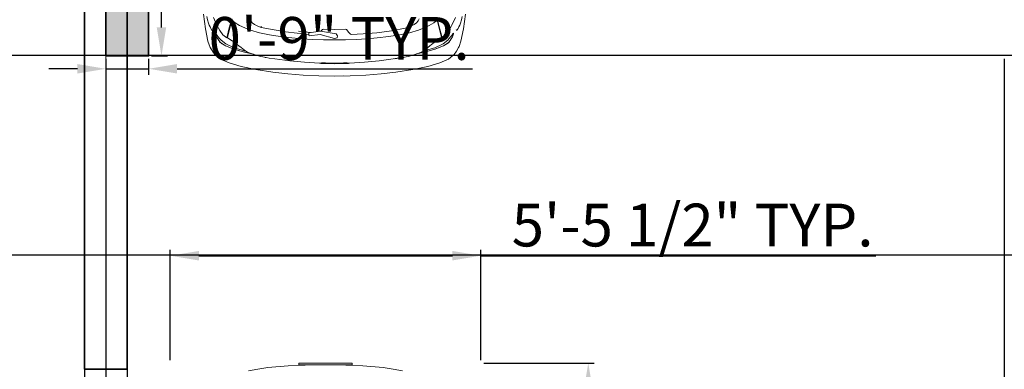
# Model space of a CAD drawing. Units: millimetres. Extents: x 595116 to 630915, y 909473 to 920225.
# Tile 113 of 134: x 629298 to 629505, y 919346 to 919419. Entities that reach past the tile are written whole.
import ezdxf

# ---------------------------------------------------------------- set-up
doc = ezdxf.new("R2010")
doc.units = ezdxf.units.MM
doc.linetypes.add('ACAD_ISO02W100', pattern=[15, 12, -3])
for name, color, linetype, lineweight in [('A-FLOR-OVHD', 253, 'ACAD_ISO02W100', 13), ('A-WALL', 1, 'Continuous', 35), ('C-PRKG-VEHI', 8, 'Continuous', 13), ('C-PROP', 7, 'Continuous', 25), ('C-PROP-REF', 240, 'ACAD_ISO02W100', 13), ('Column', 6, 'Continuous', 35), ('Dimension', 3, 'Continuous', 18)]:
    doc.layers.add(name, color=color, linetype=linetype, lineweight=lineweight)
doc.styles.get("Standard").update_dxf_attribs({"font": 'arial.ttf'})
doc.dimstyles.new('ISO-25', dxfattribs={"dimtxt": 9, "dimasz": 6, "dimexe": 1.25, "dimexo": 0.625, "dimtad": 1, "dimlunit": 4, "dimtxsty": 'Standard', "dimcen": 2.5, "dimadec": 0, "dimazin": 0, "dimtfac": 1, "dimtmove": 0, "dimatfit": 3, "dimfxl": 1, "dimarcsym": 0})

# ---------------------------------------------------------------- blocks, each defined once
blk = doc.blocks.new('A$C7ADB3080')
for p, q in [((4202.8, 1787.5), (4110.6, 1799.9)), ((4145.5, 1773.8), (4125.1, 1778.5)), ((4180, 1714.9), (4131.6, 1736.2)), ((4166.8, 1768.8), (4145.5, 1773.8)), ((4179.6, 1763.4), (4166.8, 1768.8)), ((4190.3, 1758.6), (4179.6, 1763.4)), ((4201, 1753), (4190.3, 1758.6)), ((4208.9, 1748.3), (4201, 1753)), ((4281.2, 1771.5), (4202.8, 1787.5)), ((4208.9, 1748.3), (4210.6, 1746.2)), ((4208.9, 1742.4), (4210.6, 1746.2)), ((4211.3, 1742.1), (4209, 1742.8)), ((4210, 1745), (4210.4, 1744.8)), ((4210.4, 1744.8), (4211.4, 1741.7)), ((4314.2, 1759.2), (4281.2, 1771.5)), ((4314.2, 1759.2), (4319.2, 1756.8)), ((4343.6, 1743.2), (4319.2, 1756.8)), ((4343.6, 1743.2), (4363.1, 1729.2)), ((4213.7, 1697), (4180, 1714.9)), ((4239.6, 1677.1), (4213.7, 1697)), ((4230.6, 1723.8), (4234.6, 1720.4)), ((4233.3, 1723.8), (4230.6, 1723.8)), ((4234.6, 1720.4), (4230.6, 1723.8)), ((4230.6, 1723.8), (4233.3, 1723.8)), ((4246.7, 1719.9), (4233.3, 1723.8)), ((4233.3, 1723.8), (4246.7, 1719.9)), ((4234.6, 1720.4), (4245.3, 1713.2)), ((4245.3, 1713.2), (4234.6, 1720.4)), ((4260.4, 1652.9), (4239.6, 1677.1)), ((4245.3, 1713.2), (4253.1, 1706.5)), ((4253.1, 1706.5), (4245.3, 1713.2)), ((4252.8, 1717.5), (4246.7, 1719.9)), ((4246.7, 1719.9), (4252.8, 1717.5)), ((4259.8, 1713.6), (4252.8, 1717.5)), ((4252.8, 1717.5), (4259.8, 1713.6)), ((4253.1, 1706.5), (4263.7, 1698)), ((4263.7, 1698), (4253.1, 1706.5)), ((4266.7, 1709.2), (4259.8, 1713.6)), ((4259.8, 1713.6), (4266.7, 1709.2)), ((4263.7, 1698), (4274.7, 1689.4)), ((4274.7, 1689.4), (4263.7, 1698)), ((4275.4, 1703.2), (4266.7, 1709.2)), ((4266.7, 1709.2), (4275.4, 1703.2)), ((4274.7, 1689.4), (4297.1, 1658.8)), ((4297.1, 1658.8), (4274.7, 1689.4)), ((4287.1, 1694.7), (4275.4, 1703.2)), ((4275.4, 1703.2), (4287.1, 1694.7)), ((4288.8, 1695.5), (4283, 1700)), ((4290.4, 1690), (4287.1, 1694.7)), ((4287.1, 1694.7), (4290.4, 1690)), ((4310.5, 1661.7), (4290.3, 1693.3)), ((4301.5, 1673.7), (4290.4, 1690)), ((4290.4, 1690), (4301.5, 1673.7)), ((4309.4, 1661.5), (4301.5, 1673.7)), ((4301.5, 1673.7), (4309.4, 1661.5)), ((4370.3, 1721.1), (4363.1, 1729.2)), ((4370.3, 1721.1), (4392.6, 1692.2)), ((4392.6, 1692.2), (4416.8, 1638.5)), ((4146.3, 1623.6), (4139.4, 1620.9)), ((4146.3, 1623.6), (4164.8, 1600.2)), ((4146.5, 1623.3), (4204.9, 1639.5)), ((4204.1, 1635.6), (4147.6, 1621.9)), ((4248.1, 1646.9), (4204.1, 1635.6)), ((4204.9, 1639.5), (4250.9, 1650.7)), ((4246.7, 1649.7), (4249, 1647.1)), ((4256.1, 1648.5), (4248.1, 1646.9)), ((4250.9, 1650.7), (4260.4, 1652.9)), ((4254.1, 1651.5), (4256.3, 1648.9)), ((4256.5, 1648.5), (4256.1, 1648.5)), ((4256.3, 1648.9), (4256.6, 1648.3)), ((4259.7, 1648.5), (4257.4, 1648.5)), ((4278, 1619.2), (4259.7, 1648.5)), ((4289.5, 1603), (4278, 1619.2)), ((4297.1, 1658.8), (4321.2, 1607.2)), ((4321.2, 1607.2), (4297.1, 1658.8)), ((4316, 1644.7), (4309.4, 1661.5)), ((4309.4, 1661.5), (4316, 1644.7)), ((4330.7, 1608.4), (4310.5, 1661.7)), ((4330, 1607.9), (4316, 1644.7)), ((4316, 1644.7), (4330, 1607.9)), ((4416.8, 1638.5), (4439, 1562.7)), ((4164.8, 1600.2), (4181.7, 1572.2)), ((4181.7, 1572.2), (4196.9, 1540)), ((4295.4, 1594.5), (4289.5, 1603)), ((4301.5, 1587.2), (4295.4, 1594.5)), ((4309, 1576.5), (4301.5, 1587.2)), ((4319.8, 1563.6), (4309, 1576.5)), ((4337.2, 1542.2), (4319.8, 1563.6)), ((4321.2, 1607.2), (4337.1, 1555.5)), ((4337.1, 1555.5), (4321.2, 1607.2)), ((4350.6, 1534.3), (4330, 1607.9)), ((4330, 1607.9), (4350.6, 1534.3)), ((4351.4, 1534.4), (4332.7, 1601.5)), ((4337.1, 1555.5), (4341.1, 1543)), ((4341.1, 1543), (4337.1, 1555.5)), ((4439, 1562.7), (4458.5, 1469.5)), ((4140.4, 1509.4), (4152.4, 1502.3)), ((4152.4, 1502.3), (4140.4, 1509.4)), ((4152.4, 1502.3), (4165, 1492.8)), ((4165, 1492.8), (4152.4, 1502.3)), ((4165, 1492.8), (4176.6, 1478.3)), ((4176.6, 1478.3), (4165, 1492.8)), ((4196.9, 1540), (4210.5, 1503.8)), ((4210.5, 1503.8), (4227, 1447.4)), ((4342.8, 1533.4), (4337.2, 1542.2)), ((4341.1, 1543), (4344.1, 1534.3)), ((4344.1, 1534.3), (4341.1, 1543)), ((4348.9, 1521.9), (4342.8, 1533.4)), ((4344.1, 1534.3), (4345.7, 1528.8)), ((4345.7, 1528.8), (4344.1, 1534.3)), ((4345.7, 1528.8), (4346.6, 1526.2)), ((4346.6, 1526.2), (4345.7, 1528.8)), ((4357.7, 1499.3), (4348.9, 1521.9)), ((4359.8, 1492.7), (4350.6, 1534.3)), ((4350.6, 1534.3), (4359.8, 1492.7)), ((4358.6, 1501.7), (4351.4, 1534.4)), ((4365.6, 1474.4), (4357.7, 1499.3)), ((48.4, 1460.7), (38.4, 1401.7)), ((4176.6, 1478.3), (4188.1, 1454.7)), ((4188.1, 1454.7), (4176.6, 1478.3)), ((4188.1, 1454.7), (4198, 1420.7)), ((4198, 1420.7), (4188.1, 1454.7)), ((4227, 1447.4), (4240.7, 1384.8)), ((4373.8, 1446.9), (4365.6, 1474.4)), ((4376, 1438.7), (4373.8, 1446.9)), ((4379.1, 1427.3), (4376, 1438.7)), ((4381.9, 1416.3), (4379.1, 1427.3)), ((4474.9, 1362.7), (4458.5, 1469.5)), ((27.8, 1338.5), (38.4, 1401.7)), ((4198, 1420.7), (4214.9, 1335.7)), ((4214.9, 1335.7), (4198, 1420.7)), ((4240.7, 1384.8), (4251.7, 1317)), ((4382.9, 1411.3), (4381.9, 1416.3)), ((4383.8, 1405.1), (4382.9, 1411.3)), ((4383.4, 1394.3), (4391.4, 1346)), ((4385.2, 1397), (4383.8, 1405.1)), ((4386.9, 1387.2), (4385.2, 1397)), ((4386.9, 1387.2), (4390.5, 1351.5)), ((4485.4, 1269.9), (4474.9, 1362.7)), ((27.8, 1338.5), (17, 1210.7)), ((4214.9, 1335.7), (4227, 1242)), ((4227, 1242), (4214.9, 1335.7)), ((4251.7, 1317), (4260.1, 1244.8)), ((4391.4, 1346), (4403.4, 1257.3)), ((4227, 1242), (4233.9, 1156.3)), ((4233.9, 1156.3), (4227, 1242)), ((4260.1, 1244.8), (4265.5, 1180.1)), ((4403.4, 1257.3), (4412.5, 1164.9)), ((4493.2, 1173.2), (4485.4, 1269.9)), ((17, 1210.7), (13, 1104.1)), ((4265.5, 1180.1), (4269.2, 1113.4)), ((0, 1141.1), (0, 1143.7)), ((0, 1143.7), (10.2, 1143.5)), ((0, 1136.6), (0, 1141.1)), ((0, 1131), (0, 1136.6)), ((0, 821.3), (0, 1131)), ((10.2, 1143.5), (10.2, 1140.7)), ((10.2, 1140.9), (10.2, 1143.5)), ((10.2, 1136.4), (10.2, 1140.9)), ((10.2, 1140.7), (10.2, 1136)), ((10.2, 1131.1), (10.2, 1136.4)), ((10.2, 1136), (10.2, 1130.9)), ((10.2, 821.4), (10.2, 1131.1)), ((10.2, 1130.9), (10.2, 821.4)), ((4233.9, 1156.3), (4237.4, 1081.3)), ((4237.4, 1081.3), (4233.9, 1156.3)), ((4412.5, 1164.9), (4418.1, 1070.5)), ((4498.2, 1074.5), (4493.2, 1173.2)), ((13, 1104.1), (11.7, 976.2)), ((4225.5, 1067.1), (4207.4, 1051.7)), ((4207.4, 1051.7), (4225.5, 1067.1)), ((4235.5, 1076.1), (4225.5, 1067.1)), ((4225.5, 1067.1), (4235.5, 1076.1)), ((4237.4, 1081.3), (4235.5, 1076.1)), ((4235.5, 1076.1), (4237.4, 1081.3)), ((4269.2, 1113.4), (4271.3, 1045.3)), ((4417.1, 1050.5), (4417.4, 1056.8)), ((4417.4, 1054.8), (4417.1, 1048.9)), ((4417.4, 1056.8), (4417.7, 1062.1)), ((4417.7, 1060.7), (4417.4, 1054.8)), ((4417.7, 1062.1), (4418.2, 1065.7)), ((4418.4, 1065.3), (4417.7, 1060.7)), ((4418.1, 1070.5), (4418.2, 1066)), ((4418.2, 1065.7), (4418.2, 1066)), ((4420.5, 1062.9), (4418.4, 1065.3)), ((4420.5, 1062.9), (4421, 1047.5)), ((4499.9, 976.2), (4498.2, 1074.5)), ((4207.4, 1051.7), (4204.9, 1046.5)), ((4204.9, 1046.5), (4207.4, 1051.7)), ((4204.9, 1046.5), (4206.1, 976.2)), ((4206.1, 976.2), (4204.9, 1046.5)), ((4247.3, 994.5), (4234.9, 986.8)), ((4247.3, 994.5), (4259.3, 994)), ((4259.3, 994), (4263.7, 976.4)), ((4271.3, 1045.3), (4272, 976.2)), ((4417, 1042.8), (4417.1, 1050.5)), ((4417.1, 1048.9), (4417, 1042.1)), ((4417.1, 1033.3), (4417, 1042.8)), ((4418.2, 976.2), (4417.1, 1033.3)), ((4421, 1047.5), (4421.4, 1033.2)), ((4422.2, 976.2), (4421.4, 1033.2)), ((4500, 976.2), (4498.9, 1032.6)), ((11.7, 976.2), (13, 848.2)), ((4206.1, 976.2), (4204.9, 905.9)), ((4204.9, 905.9), (4206.1, 976.2)), ((4234.9, 986.8), (4217.4, 887.5)), ((4263.7, 976.4), (4238.2, 886.7)), ((4272, 976.2), (4271.3, 907.1)), ((4417.1, 919.1), (4418.2, 976.2)), ((4421.4, 919.2), (4422.2, 976.2)), ((4498.2, 877.8), (4500, 976.2)), ((4204.9, 905.9), (4207.4, 900.7)), ((4207.4, 900.7), (4204.9, 905.9)), ((4207.4, 900.7), (4218.1, 891.5)), ((4218.1, 891.5), (4207.4, 900.7)), ((4217.4, 887.5), (4228.4, 814.6)), ((4238.2, 886.7), (4246.8, 816.9)), ((4271.3, 907.1), (4269.2, 839)), ((4418.1, 881.9), (4412.5, 787.5)), ((4417, 909.5), (4417.1, 919.1)), ((4417, 910.2), (4417.1, 903.4)), ((4417.1, 901.9), (4417, 909.5)), ((4417.1, 903.4), (4417.4, 897.5)), ((4417.4, 895.6), (4417.1, 901.9)), ((4417.4, 897.5), (4417.7, 892.2)), ((4417.7, 890.3), (4417.4, 895.6)), ((4417.7, 892.2), (4418.4, 887.1)), ((4418.2, 886.7), (4417.7, 890.3)), ((4418.2, 886.4), (4418.1, 881.9)), ((4418.2, 886.4), (4418.2, 886.7)), ((4418.4, 887.1), (4420.5, 889.6)), ((4421, 904.9), (4420.5, 889.6)), ((4421.4, 919.2), (4421, 904.9)), ((4493.2, 779.2), (4498.2, 877.8)), ((0, 816.5), (0, 821.3)), ((0, 812), (0, 816.5)), ((0, 808.8), (0, 812)), ((0, 808.8), (10.2, 808.8)), ((0, 808.8), (10.2, 808.7)), ((10.2, 816.5), (10.2, 821.4)), ((10.2, 821.4), (10.2, 816)), ((10.2, 811.8), (10.2, 816.5)), ((10.2, 816), (10.2, 811.6)), ((10.2, 808.8), (10.2, 811.8)), ((10.2, 811.6), (10.2, 808.7)), ((10.2, 808.7), (10.2, 808.8)), ((13, 848.2), (17, 741.7)), ((4226.9, 824.6), (4217.1, 750.8)), ((4221.8, 668.4), (4237.6, 814.2)), ((4228.4, 814.6), (4240.3, 814.1)), ((4246.8, 816.9), (4240.3, 814.1)), ((4269.2, 839), (4265.5, 772.3)), ((4265.5, 772.3), (4260.1, 707.5)), ((4412.5, 787.5), (4403.4, 695.1)), ((4485.4, 682.5), (4493.2, 779.2)), ((17, 741.7), (27.8, 613.9)), ((4260.1, 707.5), (4251.7, 635.4)), ((4403.4, 695.1), (4390.5, 600.8)), ((4474.9, 589.7), (4485.4, 682.5)), ((4195.1, 515.6), (4221.8, 668.4)), ((4251.7, 635.4), (4240.7, 567.6)), ((38.4, 550.7), (27.8, 613.9)), ((4240.7, 567.6), (4227, 505)), ((4386.9, 565.1), (4383.8, 547.2)), ((4390.5, 600.8), (4386.9, 565.1)), ((4458.5, 482.9), (4474.9, 589.7)), ((38.4, 550.7), (48.4, 491.6)), ((4188.1, 497.7), (4176.6, 474.1)), ((4176.6, 474.1), (4188.1, 497.7)), ((4188.8, 516.1), (4187.1, 516.4)), ((4193.4, 515.7), (4188.1, 497.7)), ((4188.1, 497.7), (4193.4, 515.7)), ((4195.1, 515.6), (4188.8, 516.1)), ((4198, 531.7), (4197.9, 531.2)), ((4197.9, 531.2), (4198, 531.7)), ((4227, 505), (4210.5, 448.6)), ((4365.6, 477.9), (4373.8, 505.4)), ((4373.8, 505.4), (4376, 513.6)), ((4376, 513.6), (4379.1, 525.1)), ((4379.1, 525.1), (4381.9, 536.1)), ((4381.9, 536.1), (4382.9, 541.1)), ((4382.9, 541.1), (4383.8, 547.2)), ((4152.4, 450), (4140.4, 443)), ((4140.4, 443), (4152.4, 450)), ((4165, 459.6), (4152.4, 450)), ((4152.4, 450), (4165, 459.6)), ((4176.6, 474.1), (4165, 459.6)), ((4165, 459.6), (4176.6, 474.1)), ((4210.5, 448.6), (4196.9, 412.4)), ((4348.9, 430.5), (4357.7, 453.1)), ((4359.8, 459.6), (4350.6, 418.1)), ((4350.6, 418.1), (4359.8, 459.6)), ((4351.4, 418), (4362.3, 467.4)), ((4357.7, 453.1), (4365.6, 477.9)), ((4458.5, 482.9), (4439, 389.6)), ((4181.7, 380.2), (4164.8, 352.2)), ((4196.9, 412.4), (4181.7, 380.2)), ((4301.5, 365.2), (4309, 375.9)), ((4309, 375.9), (4319.8, 388.8)), ((4319.8, 388.8), (4337.2, 410.2)), ((4321.2, 345.1), (4337.1, 396.9)), ((4337.1, 396.9), (4321.2, 345.1)), ((4350.6, 418.1), (4330, 344.4)), ((4330, 344.4), (4350.6, 418.1)), ((4337.1, 396.9), (4341.1, 409.4)), ((4341.1, 409.4), (4337.1, 396.9)), ((4337.2, 410.2), (4342.8, 419)), ((4338.2, 370.6), (4351.4, 418)), ((4341.1, 409.4), (4344.1, 418.1)), ((4344.1, 418.1), (4341.1, 409.4)), ((4342.8, 419), (4348.9, 430.5)), ((4344.1, 418.1), (4345.7, 423.6)), ((4345.7, 423.6), (4344.1, 418.1)), ((4345.7, 423.6), (4346.6, 426.1)), ((4346.6, 426.1), (4345.7, 423.6)), ((4439, 389.6), (4416.8, 313.9)), ((4139.4, 331.5), (4146.3, 328.7)), ((4164.8, 352.2), (4146.3, 328.7)), ((4204.9, 312.9), (4146.6, 329.1)), ((4147.7, 330.5), (4204.1, 316.7)), ((4204.1, 316.7), (4248.1, 305.5)), ((4250.9, 301.7), (4204.9, 312.9)), ((4259.7, 303.9), (4278, 333.2)), ((4278, 333.2), (4289.5, 349.4)), ((4289.5, 349.4), (4295.4, 357.9)), ((4295.4, 357.9), (4301.5, 365.2)), ((4297.1, 293.6), (4321.2, 345.1)), ((4321.2, 345.1), (4297.1, 293.6)), ((4310.5, 290.6), (4330.7, 343.8)), ((4330, 344.4), (4316, 307.6)), ((4316, 307.6), (4330, 344.4)), ((4416.8, 313.9), (4392.6, 260.2)), ((4180, 237.5), (4213.7, 255.4)), ((4213.7, 255.4), (4239.6, 275.2)), ((4239.6, 275.2), (4260.4, 299.4)), ((4249, 305.3), (4246.7, 302.7)), ((4248.1, 305.5), (4256.1, 303.9)), ((4260.4, 299.4), (4250.9, 301.7)), ((4253.1, 245.9), (4263.7, 254.4)), ((4263.7, 254.4), (4253.1, 245.9)), ((4256.3, 303.5), (4254.1, 300.9)), ((4256.1, 303.9), (4256.5, 303.9)), ((4256.6, 304.1), (4256.3, 303.5)), ((4257.4, 303.9), (4259.7, 303.9)), ((4263.7, 254.4), (4274.7, 262.9)), ((4274.7, 262.9), (4263.7, 254.4)), ((4275.4, 249.2), (4266.7, 243.2)), ((4266.7, 243.2), (4275.4, 249.2)), ((4274.7, 262.9), (4297.1, 293.6)), ((4297.1, 293.6), (4274.7, 262.9)), ((4287.1, 257.7), (4275.4, 249.2)), ((4275.4, 249.2), (4287.1, 257.7)), ((4290.4, 262.4), (4287.1, 257.7)), ((4287.1, 257.7), (4290.4, 262.4)), ((4287.4, 255.8), (4288.8, 256.8)), ((4301.5, 278.7), (4290.4, 262.4)), ((4290.4, 262.4), (4301.5, 278.7)), ((4294, 264.8), (4310.5, 290.6)), ((4309.4, 290.9), (4301.5, 278.7)), ((4301.5, 278.7), (4309.4, 290.9)), ((4316, 307.6), (4309.4, 290.9)), ((4309.4, 290.9), (4316, 307.6)), ((4392.6, 260.2), (4370.3, 231.3)), ((4131.6, 216.2), (4180, 237.5)), ((4166.8, 183.6), (4179.6, 189)), ((4179.6, 189), (4190.3, 193.8)), ((4190.3, 193.8), (4201, 199.3)), ((4201, 199.3), (4208.9, 204)), ((4210.6, 206.2), (4208.9, 209.9)), ((4210.6, 206.2), (4208.9, 204)), ((4209.1, 209.5), (4211.3, 210.3)), ((4210.4, 207.6), (4210, 207.4)), ((4211.4, 210.7), (4210.4, 207.6)), ((4230.6, 228.5), (4234.6, 232)), ((4234.6, 232), (4230.6, 228.5)), ((4233.3, 228.6), (4230.6, 228.5)), ((4230.6, 228.5), (4233.3, 228.6)), ((4246.7, 232.5), (4233.3, 228.6)), ((4233.3, 228.6), (4246.7, 232.5)), ((4234.6, 232), (4245.3, 239.2)), ((4245.3, 239.2), (4234.6, 232)), ((4245.3, 239.2), (4253.1, 245.9)), ((4253.1, 245.9), (4245.3, 239.2)), ((4252.8, 234.9), (4246.7, 232.5)), ((4246.7, 232.5), (4252.8, 234.9)), ((4259.8, 238.8), (4252.8, 234.9)), ((4252.8, 234.9), (4259.8, 238.8)), ((4266.7, 243.2), (4259.8, 238.8)), ((4259.8, 238.8), (4266.7, 243.2)), ((4281.2, 180.9), (4319.2, 195.6)), ((4314.2, 193.2), (4296.1, 186.6)), ((4319.2, 195.6), (4314.2, 193.2)), ((4319.2, 195.6), (4363.1, 223.2)), ((4343.6, 209.1), (4323.2, 198.1)), ((4363.1, 223.2), (4343.6, 209.1)), ((4363.1, 223.2), (4370.3, 231.3)), ((4110.6, 152.5), (4202.8, 164.9)), ((4125.1, 173.9), (4145.5, 178.6)), ((4145.5, 178.6), (4166.8, 183.6)), ((4202.8, 164.9), (4281.2, 180.9))]:
    blk.add_line(p, q)
blk = doc.blocks.new('*D128')
at = {"layer": 'Defpoints', "color": 0, "transparency": 16777216}
for p in [(629311.54, 920089.43), (629282.4, 919141.93), (629311.54, 919141.93)]:
    blk.add_point(p, dxfattribs=at)
at = {"layer": 'Dimension', "color": 0, "lineweight": -2, "transparency": 16777216}
for p, q in [((629310.92, 920089.43), (629281.15, 920089.43)), ((629282.4, 920083.43), (629282.4, 919147.93)), ((629310.92, 919141.93), (629281.15, 919141.93))]:
    blk.add_line(p, q, dxfattribs=at)
at = {"layer": 'Dimension', "color": 0, "transparency": 16777216}
for points in [[(629281.4, 920083.43), (629283.4, 920083.43), (629282.4, 920089.43)], [(629281.4, 919147.93), (629283.4, 919147.93), (629282.4, 919141.93)]]:
    blk.add_solid(points, dxfattribs=at)
at = {"layer": 'Dimension', "color": 0, "transparency": 16777216, "insert": (629271.16, 919615.68), "char_height": 9, "attachment_point": 5, "rotation": 90}
blk.add_mtext('78\'-11{\\H1x;\\S1/2;}"', dxfattribs=at)
blk = doc.blocks.new('COLUMN-RECT-9X18')
h = blk.add_hatch(color=256)
h.dxf.hatch_style = 1
h.paths.add_polyline_path([(9, 18), (0, 18), (0, 0), (9, 0)])
blk.add_lwpolyline([(0, 18), (9, 18), (9, 0), (0, 0)], close=True)
blk = doc.blocks.new('*D152')
at = {"layer": 'Defpoints', "color": 0, "transparency": 16777216}
for p in [(629325.04, 919429.83), (629327.74, 919429.83), (629325.04, 919411.83)]:
    blk.add_point(p, dxfattribs=at)
at = {"layer": 'Dimension', "color": 0, "lineweight": -2, "transparency": 16777216}
for p, q in [((629327.74, 919429.83), (629327.74, 919524.67)), ((629325.67, 919429.83), (629328.99, 919429.83)), ((629327.74, 919417.83), (629327.74, 919423.83)), ((629325.67, 919411.83), (629328.99, 919411.83))]:
    blk.add_line(p, q, dxfattribs=at)
at = {"layer": 'Dimension', "color": 0, "transparency": 16777216}
for points in [[(629326.74, 919423.83), (629328.74, 919423.83), (629327.74, 919429.83)], [(629326.74, 919417.83), (629328.74, 919417.83), (629327.74, 919411.83)]]:
    blk.add_solid(points, dxfattribs=at)
at = {"layer": 'Dimension', "color": 0, "transparency": 16777216, "insert": (629322.46, 919480.25), "char_height": 9, "attachment_point": 5, "rotation": 90}
blk.add_mtext('COL. 1\'-6" TYP.', dxfattribs=at)
blk = doc.blocks.new('*D153')
at = {"layer": 'Defpoints', "color": 0, "transparency": 16777216}
for p in [(629316.04, 919411.83), (629325.04, 919411.83), (629325.04, 919409.13)]:
    blk.add_point(p, dxfattribs=at)
at = {"layer": 'Dimension', "color": 0, "lineweight": -2, "transparency": 16777216}
for p, q in [((629316.04, 919411.2), (629316.04, 919407.88)), ((629325.04, 919411.2), (629325.04, 919407.88)), ((629310.04, 919409.13), (629304.04, 919409.13)), ((629316.04, 919409.13), (629325.04, 919409.13)), ((629331.04, 919409.13), (629393.15, 919409.13))]:
    blk.add_line(p, q, dxfattribs=at)
at = {"layer": 'Dimension', "color": 0, "transparency": 16777216}
for points in [[(629310.04, 919410.13), (629310.04, 919408.13), (629316.04, 919409.13)], [(629331.04, 919410.13), (629331.04, 919408.13), (629325.04, 919409.13)]]:
    blk.add_solid(points, dxfattribs=at)
at = {"layer": 'Dimension', "color": 0, "transparency": 16777216, "insert": (629365.1, 919414.35), "char_height": 9, "attachment_point": 5}
blk.add_mtext('0\'-9" TYP.', dxfattribs=at)
blk = doc.blocks.new('*D186')
at = {"layer": 'Defpoints', "color": 0, "transparency": 16777216}
for p in [(629394.93, 919347.24), (629394.93, 919196.66), (629417.52, 919196.66)]:
    blk.add_point(p, dxfattribs=at)
at = {"layer": 'Dimension', "color": 0, "lineweight": -2, "transparency": 16777216}
for p, q in [((629395.55, 919347.24), (629418.77, 919347.24)), ((629417.52, 919341.24), (629417.52, 919202.66)), ((629395.55, 919196.66), (629418.77, 919196.66))]:
    blk.add_line(p, q, dxfattribs=at)
at = {"layer": 'Dimension', "color": 0, "transparency": 16777216}
for points in [[(629416.52, 919341.24), (629418.52, 919341.24), (629417.52, 919347.24)], [(629416.52, 919202.66), (629418.52, 919202.66), (629417.52, 919196.66)]]:
    blk.add_solid(points, dxfattribs=at)
at = {"layer": 'Dimension', "color": 0, "transparency": 16777216, "insert": (629412.24, 919271.95), "char_height": 9, "attachment_point": 5, "rotation": 90}
blk.add_mtext('CAR 12\'-6 1/2" TYP.', dxfattribs=at)
blk = doc.blocks.new('*D187')
at = {"layer": 'Defpoints', "color": 0, "transparency": 16777216}
for p in [(629394.93, 919369.82), (629329.6, 919347.24), (629394.93, 919347.24)]:
    blk.add_point(p, dxfattribs=at)
at = {"layer": 'Dimension', "color": 0, "lineweight": -2, "transparency": 16777216}
for p, q in [((629329.6, 919347.86), (629329.6, 919371.07)), ((629394.93, 919347.86), (629394.93, 919371.07)), ((629335.6, 919369.82), (629388.93, 919369.82)), ((629394.93, 919369.82), (629478.01, 919369.82))]:
    blk.add_line(p, q, dxfattribs=at)
at = {"layer": 'Dimension', "color": 0, "transparency": 16777216}
for points in [[(629335.6, 919370.82), (629335.6, 919368.82), (629329.6, 919369.82)], [(629388.93, 919370.82), (629388.93, 919368.82), (629394.93, 919369.82)]]:
    blk.add_solid(points, dxfattribs=at)
at = {"layer": 'Dimension', "color": 0, "transparency": 16777216, "insert": (629439.47, 919375.1), "char_height": 9, "attachment_point": 5}
blk.add_mtext('5\'-5 1/2" TYP.', dxfattribs=at)
blk = doc.blocks.new('*D215')
at = {"layer": 'Defpoints', "color": 0, "transparency": 16777216}
for p in [(629316.04, 919411.83), (629505.04, 919411.83), (629505.04, 918832.38)]:
    blk.add_point(p, dxfattribs=at)
at = {"layer": 'Dimension', "color": 0, "lineweight": -2, "transparency": 16777216}
for p, q in [((629316.04, 919411.2), (629316.04, 918831.13)), ((629505.04, 919411.2), (629505.04, 918831.13)), ((629322.04, 918832.38), (629499.04, 918832.38))]:
    blk.add_line(p, q, dxfattribs=at)
at = {"layer": 'Dimension', "color": 0, "transparency": 16777216}
for points in [[(629322.04, 918833.38), (629322.04, 918831.38), (629316.04, 918832.38)], [(629499.04, 918833.38), (629499.04, 918831.38), (629505.04, 918832.38)]]:
    blk.add_solid(points, dxfattribs=at)
at = {"layer": 'Dimension', "color": 0, "transparency": 16777216, "insert": (629410.54, 918837.6), "char_height": 9, "attachment_point": 5}
blk.add_mtext('15\'-9"', dxfattribs=at)
blk = doc.blocks.new('*D216')
at = {"layer": 'Defpoints', "color": 0, "transparency": 16777216}
for p in [(629505.04, 919411.83), (629743.54, 919411.93), (629743.54, 918832.38)]:
    blk.add_point(p, dxfattribs=at)
at = {"layer": 'Dimension', "color": 0, "lineweight": -2, "transparency": 16777216}
for p, q in [((629505.04, 919411.2), (629505.04, 918831.13)), ((629743.54, 919411.3), (629743.54, 918831.13)), ((629511.04, 918832.38), (629737.54, 918832.38))]:
    blk.add_line(p, q, dxfattribs=at)
at = {"layer": 'Dimension', "color": 0, "transparency": 16777216}
for points in [[(629511.04, 918833.38), (629511.04, 918831.38), (629505.04, 918832.38)], [(629737.54, 918833.38), (629737.54, 918831.38), (629743.54, 918832.38)]]:
    blk.add_solid(points, dxfattribs=at)
at = {"layer": 'Dimension', "color": 0, "transparency": 16777216, "insert": (629624.29, 918837.66), "char_height": 9, "attachment_point": 5}
blk.add_mtext('19\'-10 1/2"', dxfattribs=at)
blk = doc.blocks.new('*D217')
at = {"layer": 'Defpoints', "color": 0, "transparency": 16777216}
for p in [(629743.54, 919411.93), (629155.38, 919369.93), (629743.54, 919369.93)]:
    blk.add_point(p, dxfattribs=at)
at = {"layer": 'Dimension', "color": 0, "lineweight": -2, "transparency": 16777216}
for p, q in [((629742.92, 919411.93), (629154.13, 919411.93)), ((629155.38, 919405.93), (629155.38, 919375.93)), ((629742.92, 919369.93), (629154.13, 919369.93))]:
    blk.add_line(p, q, dxfattribs=at)
at = {"layer": 'Dimension', "color": 0, "transparency": 16777216}
for points in [[(629154.38, 919405.93), (629156.38, 919405.93), (629155.38, 919411.93)], [(629154.38, 919375.93), (629156.38, 919375.93), (629155.38, 919369.93)]]:
    blk.add_solid(points, dxfattribs=at)
at = {"layer": 'Dimension', "color": 0, "transparency": 16777216, "insert": (629150.16, 919390.93), "char_height": 9, "attachment_point": 5, "rotation": 90}
blk.add_mtext('3\'-6"', dxfattribs=at)

msp = doc.modelspace()

# ---------------------------------------------------------------- linework, layer by layer
at = {"layer": 'A-FLOR-OVHD'}
msp.add_line((629505.041, 919369.928), (629320.541, 919369.928), dxfattribs=at)
at = {"layer": 'A-WALL'}
for p, q in [((629320.541, 919345.928), (629320.541, 919957.928)), ((629311.541, 919345.928), (629320.541, 919345.928))]:
    msp.add_line(p, q, dxfattribs=at)
msp.add_lwpolyline([(629311.541, 919345.928), (629311.541, 919957.928)], dxfattribs=at)
at = {"layer": 'C-PROP'}
for p, q in [((629311.541, 919345.928), (629311.541, 919141.928)), ((629320.541, 919345.928), (629320.541, 919150.928))]:
    msp.add_line(p, q, dxfattribs=at)
at = {"layer": 'C-PROP-REF'}
msp.add_line((629316.041, 919146.428), (629316.041, 920084.928), dxfattribs=at)

# ---------------------------------------------------------------- block references
at = {"layer": 'C-PRKG-VEHI', "xscale": 0.0334614614063694, "yscale": 0.0334614614063694, "zscale": 0.0334614614063694, "rotation": 270}
for p in [(629331.465, 919558.166), (629329.6, 919347.236)]:
    msp.add_blockref('A$C7ADB3080', p, dxfattribs=at)
at = {"layer": 'Column'}
msp.add_blockref('COLUMN-RECT-9X18', (629316.041, 919411.828), dxfattribs=at)

# ---------------------------------------------------------------- dimensions: what is measured, and where the dimension line sits
at = {"layer": 'Dimension'}
for base, p1, p2, override, picture, middle in [((629282.395, 919141.928), (629311.541, 920089.428), (629311.541, 919141.928), {"dimclrd": 0, "dimclre": 0, "dimclrt": 0}, '*D128', (629271.157, 919615.678)), ((629155.382, 919369.928), (629743.541, 919411.928), (629743.541, 919369.928), {"dimdec": 1, "dimlfac": 1, "dimrnd": 0, "dimzin": 1, "dimdsep": 46, "dimlunit": 4, "dimfrac": 2}, '*D217', (629150.159, 919390.928))]:
    dim = msp.add_linear_dim(base=base, p1=p1, p2=p2, angle=90, dimstyle='ISO-25', override=override, dxfattribs=at)
    dim.commit()
    dim.dimension.update_dxf_attribs({"geometry": picture, "text_midpoint": middle})
for base, p1, p2, angle, text, picture, middle in [((629327.741, 919429.828), (629325.041, 919411.828), (629325.041, 919429.828), 90, 'COL. <> TYP.', '*D152', (629322.459, 919480.25)), ((629417.516, 919196.66), (629394.93, 919347.236), (629394.93, 919196.66), 270, 'CAR <> TYP.', '*D186', (629412.238, 919271.948))]:
    dim = msp.add_linear_dim(base=base, p1=p1, p2=p2, angle=angle, text=text, dimstyle='ISO-25', override={"dimdec": 1, "dimlfac": 1, "dimrnd": 0, "dimzin": 1, "dimdsep": 46, "dimlunit": 4, "dimfrac": 2}, dxfattribs=at)
    dim.commit()
    dim.dimension.update_dxf_attribs({"geometry": picture, "text_midpoint": middle})
for base, p1, p2, picture, middle in [((629325.041, 919409.128), (629316.041, 919411.828), (629325.041, 919411.828), '*D153', (629365.096, 919414.348)), ((629394.93, 919369.823), (629329.6, 919347.236), (629394.93, 919347.236), '*D187', (629439.47, 919375.101))]:
    dim = msp.add_linear_dim(base=base, p1=p1, p2=p2, text='<> TYP.', dimstyle='ISO-25', override={"dimdec": 1, "dimlfac": 1, "dimrnd": 0, "dimzin": 1, "dimdsep": 46, "dimlunit": 4, "dimfrac": 2}, dxfattribs=at)
    dim.commit()
    dim.dimension.update_dxf_attribs({"geometry": picture, "text_midpoint": middle})
for base, p1, p2, picture, middle in [((629505.041, 918832.378), (629316.041, 919411.828), (629505.041, 919411.828), '*D215', (629410.541, 918837.598)), ((629743.541, 918832.378), (629505.041, 919411.828), (629743.541, 919411.928), '*D216', (629624.291, 918837.656))]:
    dim = msp.add_linear_dim(base=base, p1=p1, p2=p2, dimstyle='ISO-25', override={"dimdec": 1, "dimlfac": 1, "dimrnd": 0, "dimzin": 1, "dimdsep": 46, "dimlunit": 4, "dimfrac": 2}, dxfattribs=at)
    dim.commit()
    dim.dimension.update_dxf_attribs({"geometry": picture, "text_midpoint": middle})

doc.saveas('drawing.dxf')
